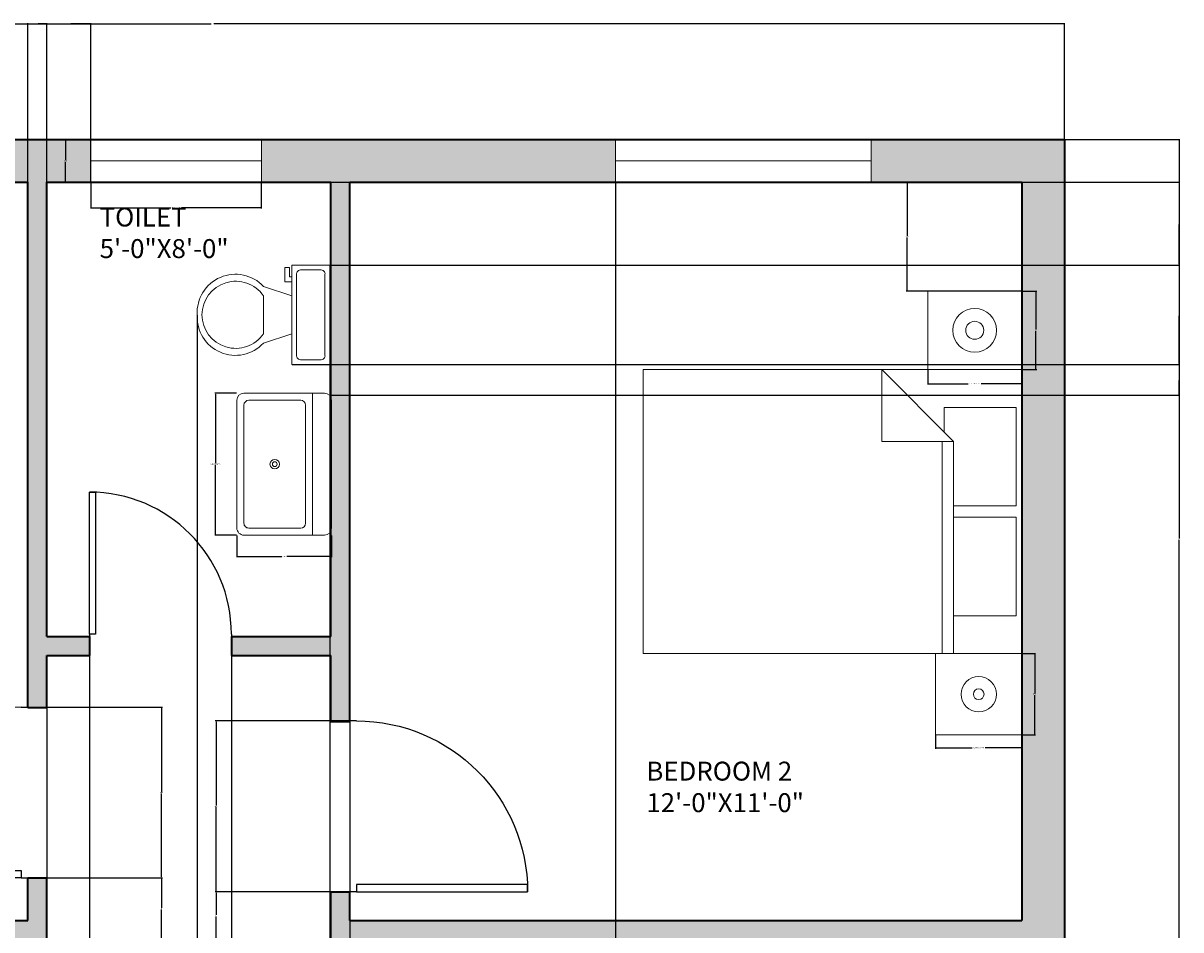
# Model space of a CAD drawing. Units: inches. Extents: x -29 to 443, y -589 to 39.
# Tile 5 of 5: x 139 to 384, y -153 to 39. Entities that reach past the tile are written whole.
import ezdxf

# ---------------------------------------------------------------- set-up
doc = ezdxf.new("R2010")
doc.units = ezdxf.units.IN
for name, color, linetype, lineweight in [('A-ANNO-DIMS', 2, 'Continuous', 18), ('A-AREA-IDEN', 7, 'Continuous', 18), ('A-DOOR', 3, 'Continuous', 25), ('A-FLOR-FIXT', 9, 'Continuous', 18), ('A-FURN', 9, 'Continuous', 18), ('A-GLAZ', 4, 'Continuous', 18), ('A-WALL', 7, 'Continuous', 35)]:
    doc.layers.add(name, color=color, linetype=linetype, lineweight=lineweight)
doc.layers.add('A-WALL-PATT', color=251, linetype='Continuous', lineweight=13, true_color=0x636466)
doc.styles.get("Standard").update_dxf_attribs({"font": 'arial.ttf'})
doc.dimstyles.get("Standard").update_dxf_attribs({"dimtxt": 0.18, "dimasz": 0.18, "dimexe": 0.18, "dimexo": 0.0625, "dimgap": 0.09, "dimtad": 0, "dimtih": 1, "dimtoh": 1, "dimdec": 4, "dimzin": 0, "dimdsep": 46, "dimtxsty": 'Standard', "dimcen": 0.09, "dimadec": 0, "dimazin": 0, "dimtfac": 1, "dimtdec": 4, "dimtofl": 0, "dimtmove": 0, "dimatfit": 3, "dimfxl": 1, "dimtolj": 1, "dimtzin": 0, "dimarcsym": 0})

# ---------------------------------------------------------------- blocks, each defined once
blk = doc.blocks.new('*U3')
for p, q in [((0, 0), (0, -6)), ((40, 0), (40, -6))]:
    blk.add_line(p, q)
blk.add_lwpolyline([(0, 0), (0, 40), (1.75, 40), (1.75, 0)], close=True)
blk.add_arc((0, 0), 40, 0, 90)
blk = doc.blocks.new('Sink-single - 30 in top')
blk.add_line((-15, -3.999996), (15, -3.999996))
for points in [[(-13.5, 0), (13.5, 0)], [(-15, -18.499996), (-15, -1.5)], [(15, -1.5), (15, -18.499996)], [(-13.5, -17.499996), (-13.5, -6.499996)], [(-12.5, -5.499996), (12.5, -5.499996)], [(13.5, -6.499996), (13.5, -17.499996)], [(12.5, -18.499996), (-12.5, -18.499996)], [(13.5, -19.999996), (-13.5, -19.999996)]]:
    blk.add_lwpolyline(points)
for radius in [1, 0.5]:
    blk.add_circle((0, -11.999996), radius)
for centre, radius, start, end in [((-13.5, -1.5), 1.5, 90, 180), ((13.5, -1.5), 1.5, 0, 90), ((-12.5, -6.499996), 1, 90, 180), ((12.5, -6.499996), 1, 0, 90), ((-13.5, -18.499996), 1.5, 180, 270), ((-12.5, -17.499996), 1, 180, 270), ((12.5, -17.499996), 1, 270, 0), ((13.5, -18.499996), 1.5, 270, 0)]:
    blk.add_arc(centre, radius, start, end)
blk = doc.blocks.new('Bed - Queen')
for p, q in [((0, -80.00003), (0, 0)), ((0, 0), (59.99999, 0)), ((59.99999, 0), (59.99999, -80.00003)), ((7.99999, -1.2), (28.79998, -1.2)), ((7.99999, -14.4), (7.99999, -1.2)), ((28.79998, -1.2), (28.79998, -14.4)), ((31.19999, -1.2), (51.99999, -1.2)), ((31.19999, -14.4), (31.19999, -1.2)), ((51.99999, -1.2), (51.99999, -16.4)), ((0, -14.4), (44.8, -14.4)), ((59.99999, -29.6), (44.8, -14.4)), ((44.8, -14.4), (44.8, -29.6)), ((44.8, -16.8), (0, -16.8)), ((51.99999, -16.4), (46.79936, -16.4)), ((44.8, -29.6), (59.99999, -29.6)), ((59.99999, -80.00003), (0, -80.00003))]:
    blk.add_line(p, q)
blk = doc.blocks.new('*U9')
for p, q in [((9.5, -6), (9.5, -2)), ((-10, -8.5), (-8, -8.5)), ((-10, -9.5), (-10, -8.5)), ((-7, -9.5), (-10, -9.5)), ((-8, -8.5), (-8, -8)), ((-7, -8), (-7, -9.5)), ((-4, -8), (-6, -14)), ((4, -8), (6, -14)), ((4, -14), (-4, -14))]:
    blk.add_line(p, q)
blk.add_lwpolyline([(10.5, -8), (10.5, 0), (-10.5, 0), (-10.5, -8)], close=True)
for points in [[(-9.5, -2), (-9.5, -6)], [(8.5, -1), (-8.5, -1)], [(-8.5, -7), (8.5, -7)]]:
    blk.add_lwpolyline(points)
for centre, radius, start, end in [((-8.625, -1.875), 0.8839, 81.8699, 188.1301), ((8.625, -1.875), 0.8839, 351.8699, 98.1301), ((-8.625, -6.125), 0.8839, 171.869898, 278.1301), ((8.625, -6.125), 0.8839, 261.8699, 8.1301), ((-0.4772, -19.9188), 8.0953, 133.01722, 273.38), ((0.0374, -19.8731), 7.127, 124.50543, 269.7), ((-0.0373, -19.8731), 7.127, 270.3, 55.4946), ((0.4773, -19.9188), 8.0953, 266.62, 46.9828)]:
    blk.add_arc(centre, radius, start, end)
blk = doc.blocks.new('WIN-54IN')
blk.add_line((54, 4.5), (0, 4.5))
blk.add_lwpolyline([(0, 9), (54, 9), (54, 0), (0, 0)], close=True)
blk = doc.blocks.new('WIN-36IN')
blk.add_line((4.5, 36), (4.5, 0))
blk.add_lwpolyline([(0, 0), (0, 36), (9, 36), (9, 0)], close=True)
blk = doc.blocks.new('NIGHTSTAND-LARGE')
blk.add_lwpolyline([(19.87, 0), (19.87, 16.61), (0, 16.61), (0, 0)], close=True)
for radius in [4.62, 1.9]:
    blk.add_circle((9.93, 8.31), radius)
blk = doc.blocks.new('NIGHTSTAND-SMALL')
blk.add_lwpolyline([(18.21, 17.2), (18.21, 0), (0, 0), (0, 17.2)], close=True)
for radius in [3.74, 1.13]:
    blk.add_circle((9.11, 8.6), radius)
blk = doc.blocks.new('*D22')
at = {"layer": 'A-ANNO-DIMS', "color": 0, "lineweight": -2, "transparency": 16777216}
for p, q in [((330.57, -34.29), (330.57, -37.39)), ((350.44, -34.29), (350.44, -37.39)), ((330.75, -37.21), (339.13, -37.21)), ((350.26, -37.21), (341.88, -37.21))]:
    blk.add_line(p, q, dxfattribs=at)
at = {"layer": 'A-ANNO-DIMS', "color": 0, "transparency": 16777216}
for points in [[(330.75, -37.18), (330.75, -37.24), (330.57, -37.21)], [(350.26, -37.18), (350.26, -37.24), (350.44, -37.21)]]:
    blk.add_solid(points, dxfattribs=at)
at = {"layer": 'Defpoints', "color": 0, "transparency": 16777216}
for p in [(330.57, -34.23), (350.44, -34.23), (350.44, -37.21)]:
    blk.add_point(p, dxfattribs=at)
at = {"layer": 'A-ANNO-DIMS', "color": 0, "transparency": 16777216, "insert": (340.5, -37.21), "char_height": 0.18, "attachment_point": 5}
blk.add_mtext('\\A1;NIGHTSTAND 20 TYP.', dxfattribs=at)
blk = doc.blocks.new('*D23')
at = {"layer": 'A-ANNO-DIMS', "color": 0, "lineweight": -2, "transparency": 16777216}
for p, q in [((350.5, -17.62), (353.6, -17.62)), ((353.42, -17.8), (353.42, -25.75)), ((353.42, -34.05), (353.42, -26.11)), ((350.5, -34.23), (353.6, -34.23))]:
    blk.add_line(p, q, dxfattribs=at)
at = {"layer": 'A-ANNO-DIMS', "color": 0, "transparency": 16777216}
for points in [[(353.39, -17.8), (353.45, -17.8), (353.42, -17.62)], [(353.39, -34.05), (353.45, -34.05), (353.42, -34.23)]]:
    blk.add_solid(points, dxfattribs=at)
at = {"layer": 'Defpoints', "color": 0, "transparency": 16777216}
for p in [(350.44, -17.62), (353.42, -17.62), (350.44, -34.23)]:
    blk.add_point(p, dxfattribs=at)
at = {"layer": 'A-ANNO-DIMS', "color": 0, "transparency": 16777216, "insert": (353.42, -25.93), "char_height": 0.18, "attachment_point": 5}
blk.add_mtext('\\A1;17 TYP.', dxfattribs=at)
blk = doc.blocks.new('*D24')
at = {"layer": 'A-ANNO-DIMS', "color": 0, "lineweight": -2, "transparency": 16777216}
for p, q in [((332.22, -111.49), (332.22, -114.34)), ((350.44, -111.49), (350.44, -114.34)), ((332.4, -114.16), (339.95, -114.16)), ((350.26, -114.16), (342.7, -114.16))]:
    blk.add_line(p, q, dxfattribs=at)
at = {"layer": 'A-ANNO-DIMS', "color": 0, "transparency": 16777216}
for points in [[(332.4, -114.13), (332.4, -114.19), (332.22, -114.16)], [(350.26, -114.13), (350.26, -114.19), (350.44, -114.16)]]:
    blk.add_solid(points, dxfattribs=at)
at = {"layer": 'Defpoints', "color": 0, "transparency": 16777216}
for p in [(332.22, -111.43), (350.44, -111.43), (350.44, -114.16)]:
    blk.add_point(p, dxfattribs=at)
at = {"layer": 'A-ANNO-DIMS', "color": 0, "transparency": 16777216, "insert": (341.33, -114.16), "char_height": 0.18, "attachment_point": 5}
blk.add_mtext('\\A1;NIGHTSTAND 18 TYP.', dxfattribs=at)
blk = doc.blocks.new('*D25')
at = {"layer": 'A-ANNO-DIMS', "color": 0, "lineweight": -2, "transparency": 16777216}
for p, q in [((350.5, -94.23), (353.35, -94.23)), ((353.17, -94.41), (353.17, -102.65)), ((353.17, -111.25), (353.17, -103.01)), ((350.5, -111.43), (353.35, -111.43))]:
    blk.add_line(p, q, dxfattribs=at)
at = {"layer": 'A-ANNO-DIMS', "color": 0, "transparency": 16777216}
for points in [[(353.14, -94.41), (353.2, -94.41), (353.17, -94.23)], [(353.14, -111.25), (353.2, -111.25), (353.17, -111.43)]]:
    blk.add_solid(points, dxfattribs=at)
at = {"layer": 'Defpoints', "color": 0, "transparency": 16777216}
for p in [(350.44, -94.23), (353.17, -94.23), (350.44, -111.43)]:
    blk.add_point(p, dxfattribs=at)
at = {"layer": 'A-ANNO-DIMS', "color": 0, "transparency": 16777216, "insert": (353.17, -102.83), "char_height": 0.18, "attachment_point": 5}
blk.add_mtext('\\A1;17 TYP.', dxfattribs=at)
blk = doc.blocks.new('*D26')
at = {"layer": 'A-ANNO-DIMS', "color": 0, "lineweight": -2, "transparency": 16777216}
for p, q in [((184.53, -39.21), (179.91, -39.21)), ((180.09, -39.39), (180.09, -54.03)), ((180.09, -69.03), (180.09, -54.39)), ((184.53, -69.21), (179.91, -69.21))]:
    blk.add_line(p, q, dxfattribs=at)
at = {"layer": 'A-ANNO-DIMS', "color": 0, "transparency": 16777216}
for points in [[(180.06, -39.39), (180.12, -39.39), (180.09, -39.21)], [(180.06, -69.03), (180.12, -69.03), (180.09, -69.21)]]:
    blk.add_solid(points, dxfattribs=at)
at = {"layer": 'Defpoints', "color": 0, "transparency": 16777216}
for p in [(184.59, -39.21), (180.09, -69.21), (184.59, -69.21)]:
    blk.add_point(p, dxfattribs=at)
at = {"layer": 'A-ANNO-DIMS', "color": 0, "transparency": 16777216, "insert": (180.09, -54.21), "char_height": 0.18, "attachment_point": 5}
blk.add_mtext('\\A1;BASIN TOP 30 TYP.', dxfattribs=at)
blk = doc.blocks.new('*D27')
at = {"layer": 'A-ANNO-DIMS', "color": 0, "lineweight": -2, "transparency": 16777216}
for p, q in [((184.59, -69.27), (184.59, -73.89)), ((204.59, -69.27), (204.59, -73.89)), ((184.77, -73.71), (194.06, -73.71)), ((204.41, -73.71), (195.12, -73.71))]:
    blk.add_line(p, q, dxfattribs=at)
at = {"layer": 'A-ANNO-DIMS', "color": 0, "transparency": 16777216}
for points in [[(184.77, -73.68), (184.77, -73.74), (184.59, -73.71)], [(204.41, -73.68), (204.41, -73.74), (204.59, -73.71)]]:
    blk.add_solid(points, dxfattribs=at)
at = {"layer": 'Defpoints', "color": 0, "transparency": 16777216}
for p in [(184.59, -69.21), (204.59, -69.21), (204.59, -73.71)]:
    blk.add_point(p, dxfattribs=at)
at = {"layer": 'A-ANNO-DIMS', "color": 0, "transparency": 16777216, "insert": (194.59, -73.71), "char_height": 0.18, "attachment_point": 5}
blk.add_mtext('\\A1;20 TYP.', dxfattribs=at)
blk = doc.blocks.new('*D28')
at = {"layer": 'A-ANNO-DIMS', "color": 0, "lineweight": -2, "transparency": 16777216}
for p, q in [((153.76, 5.32), (153.76, -0.19)), ((189.76, 5.32), (189.76, -0.19)), ((153.94, -0.01), (170.64, -0.01)), ((189.58, -0.01), (172.88, -0.01))]:
    blk.add_line(p, q, dxfattribs=at)
at = {"layer": 'A-ANNO-DIMS', "color": 0, "transparency": 16777216}
for points in [[(153.94, 0.02), (153.94, -0.04), (153.76, -0.01)], [(189.58, 0.02), (189.58, -0.04), (189.76, -0.01)]]:
    blk.add_solid(points, dxfattribs=at)
at = {"layer": 'Defpoints', "color": 0, "transparency": 16777216}
for p in [(153.76, 5.39), (189.76, 5.39), (189.76, -0.01)]:
    blk.add_point(p, dxfattribs=at)
at = {"layer": 'A-ANNO-DIMS', "color": 0, "transparency": 16777216, "insert": (171.76, -0.01), "char_height": 0.18, "attachment_point": 5}
blk.add_mtext('\\A1;WINDOW 36 TYP.', dxfattribs=at)
blk = doc.blocks.new('*D29')
at = {"layer": 'A-ANNO-DIMS', "color": 0, "lineweight": -2, "transparency": 16777216}
for p, q in [((153.7, 14.39), (148.18, 14.39)), ((148.36, 14.21), (148.36, 10.07)), ((148.36, 5.57), (148.36, 9.7)), ((153.7, 5.39), (148.18, 5.39))]:
    blk.add_line(p, q, dxfattribs=at)
at = {"layer": 'A-ANNO-DIMS', "color": 0, "transparency": 16777216}
for points in [[(148.33, 14.21), (148.39, 14.21), (148.36, 14.39)], [(148.33, 5.57), (148.39, 5.57), (148.36, 5.39)]]:
    blk.add_solid(points, dxfattribs=at)
at = {"layer": 'Defpoints', "color": 0, "transparency": 16777216}
for p in [(153.76, 14.39), (148.36, 5.39), (153.76, 5.39)]:
    blk.add_point(p, dxfattribs=at)
at = {"layer": 'A-ANNO-DIMS', "color": 0, "transparency": 16777216, "insert": (148.36, 9.89), "char_height": 0.18, "attachment_point": 5}
blk.add_mtext('\\A1;9 TYP.', dxfattribs=at)
blk = doc.blocks.new('*D36')
at = {"layer": 'A-ANNO-DIMS', "color": 0, "lineweight": -2, "transparency": 16777216}
for p, q in [((-0.56, 14.45), (-0.56, 38.99)), ((-0.38, 38.81), (179.15, 38.81)), ((359.26, 38.81), (179.72, 38.81)), ((359.44, 14.45), (359.44, 38.99))]:
    blk.add_line(p, q, dxfattribs=at)
at = {"layer": 'A-ANNO-DIMS', "color": 0, "transparency": 16777216}
for points in [[(-0.38, 38.84), (-0.38, 38.78), (-0.56, 38.81)], [(359.26, 38.84), (359.26, 38.78), (359.44, 38.81)]]:
    blk.add_solid(points, dxfattribs=at)
at = {"layer": 'Defpoints', "color": 0, "transparency": 16777216}
for p in [(359.44, 38.81), (-0.56, 14.39), (359.44, 14.39)]:
    blk.add_point(p, dxfattribs=at)
at = {"layer": 'A-ANNO-DIMS', "color": 0, "transparency": 16777216, "insert": (179.44, 38.81), "char_height": 0.18, "attachment_point": 5}
blk.add_mtext('\\A1;360', dxfattribs=at)
blk = doc.blocks.new('*D39')
at = {"layer": 'A-ANNO-DIMS', "color": 0, "lineweight": -2, "transparency": 16777216}
for p, q in [((144.44, 5.45), (144.44, 38.99)), ((144.62, 38.81), (148.71, 38.81)), ((153.58, 38.81), (149.49, 38.81)), ((153.76, 5.45), (153.76, 38.99))]:
    blk.add_line(p, q, dxfattribs=at)
at = {"layer": 'A-ANNO-DIMS', "color": 0, "transparency": 16777216}
for points in [[(144.62, 38.84), (144.62, 38.78), (144.44, 38.81)], [(153.58, 38.84), (153.58, 38.78), (153.76, 38.81)]]:
    blk.add_solid(points, dxfattribs=at)
at = {"layer": 'Defpoints', "color": 0, "transparency": 16777216}
for p in [(144.44, 38.81), (144.44, 5.39), (153.76, 5.39)]:
    blk.add_point(p, dxfattribs=at)
at = {"layer": 'A-ANNO-DIMS', "color": 0, "transparency": 16777216, "insert": (149.1, 38.81), "char_height": 0.18, "attachment_point": 5}
blk.add_mtext('\\A1;9.326', dxfattribs=at)
blk = doc.blocks.new('*D40')
at = {"layer": 'A-ANNO-DIMS', "color": 0, "lineweight": -2, "transparency": 16777216}
for p, q in [((208.44, 5.32), (208.44, -492.89)), ((264.58, 5.32), (264.58, -492.89)), ((208.62, -492.71), (236.11, -492.71)), ((264.4, -492.71), (236.9, -492.71))]:
    blk.add_line(p, q, dxfattribs=at)
at = {"layer": 'A-ANNO-DIMS', "color": 0, "transparency": 16777216}
for points in [[(208.62, -492.68), (208.62, -492.74), (208.44, -492.71)], [(264.4, -492.68), (264.4, -492.74), (264.58, -492.71)]]:
    blk.add_solid(points, dxfattribs=at)
at = {"layer": 'Defpoints', "color": 0, "transparency": 16777216}
for p in [(208.44, 5.39), (264.58, 5.39), (208.44, -492.71)]:
    blk.add_point(p, dxfattribs=at)
at = {"layer": 'A-ANNO-DIMS', "color": 0, "transparency": 16777216, "insert": (236.51, -492.71), "char_height": 0.18, "attachment_point": 5}
blk.add_mtext('\\A1;56.14', dxfattribs=at)
blk = doc.blocks.new('*D44')
at = {"layer": 'A-ANNO-DIMS', "color": 0, "lineweight": -2, "transparency": 16777216}
for p, q in [((359.5, 14.39), (383.85, 14.39)), ((383.67, 14.21), (383.67, -69.93)), ((383.67, -154.43), (383.67, -70.3)), ((359.5, -154.61), (383.85, -154.61))]:
    blk.add_line(p, q, dxfattribs=at)
at = {"layer": 'A-ANNO-DIMS', "color": 0, "transparency": 16777216}
for points in [[(383.64, 14.21), (383.7, 14.21), (383.67, 14.39)], [(383.64, -154.43), (383.7, -154.43), (383.67, -154.61)]]:
    blk.add_solid(points, dxfattribs=at)
at = {"layer": 'Defpoints', "color": 0, "transparency": 16777216}
for p in [(359.44, 14.39), (359.44, -154.61), (383.67, -154.61)]:
    blk.add_point(p, dxfattribs=at)
at = {"layer": 'A-ANNO-DIMS', "color": 0, "transparency": 16777216, "insert": (383.67, -70.11), "char_height": 0.18, "attachment_point": 5}
blk.add_mtext('\\A1;169', dxfattribs=at)
blk = doc.blocks.new('*D50')
at = {"layer": 'A-ANNO-DIMS', "color": 0, "lineweight": -2, "transparency": 16777216}
for p, q in [((144.5, -105.59), (168.85, -105.59)), ((168.67, -105.77), (168.67, -123.42)), ((168.67, -141.43), (168.67, -123.78)), ((144.5, -141.61), (168.85, -141.61))]:
    blk.add_line(p, q, dxfattribs=at)
at = {"layer": 'A-ANNO-DIMS', "color": 0, "transparency": 16777216}
for points in [[(168.64, -105.77), (168.7, -105.77), (168.67, -105.59)], [(168.64, -141.43), (168.7, -141.43), (168.67, -141.61)]]:
    blk.add_solid(points, dxfattribs=at)
at = {"layer": 'Defpoints', "color": 0, "transparency": 16777216}
for p in [(144.44, -105.59), (144.44, -141.61), (168.67, -141.61)]:
    blk.add_point(p, dxfattribs=at)
at = {"layer": 'A-ANNO-DIMS', "color": 0, "transparency": 16777216, "insert": (168.67, -123.6), "char_height": 0.18, "attachment_point": 5}
blk.add_mtext('\\A1;36.03', dxfattribs=at)
blk = doc.blocks.new('*D51')
at = {"layer": 'A-ANNO-DIMS', "color": 0, "lineweight": -2, "transparency": 16777216}
for p, q in [((144.5, -141.61), (168.85, -141.61)), ((168.67, -141.79), (168.67, -147.93)), ((168.67, -154.43), (168.67, -148.3)), ((144.5, -154.61), (168.85, -154.61))]:
    blk.add_line(p, q, dxfattribs=at)
at = {"layer": 'A-ANNO-DIMS', "color": 0, "transparency": 16777216}
for points in [[(168.64, -141.79), (168.7, -141.79), (168.67, -141.61)], [(168.64, -154.43), (168.7, -154.43), (168.67, -154.61)]]:
    blk.add_solid(points, dxfattribs=at)
at = {"layer": 'Defpoints', "color": 0, "transparency": 16777216}
for p in [(144.44, -141.61), (144.44, -154.61), (168.67, -154.61)]:
    blk.add_point(p, dxfattribs=at)
at = {"layer": 'A-ANNO-DIMS', "color": 0, "transparency": 16777216, "insert": (168.67, -148.11), "char_height": 0.18, "attachment_point": 5}
blk.add_mtext('\\A1;13', dxfattribs=at)
blk = doc.blocks.new('*D52')
at = {"layer": 'A-ANNO-DIMS', "color": 0, "lineweight": -2, "transparency": 16777216}
for p, q in [((153.44, -94.68), (153.44, -492.89)), ((183.44, -94.68), (183.44, -492.89)), ((153.62, -492.71), (168.22, -492.71)), ((183.26, -492.71), (168.65, -492.71))]:
    blk.add_line(p, q, dxfattribs=at)
at = {"layer": 'A-ANNO-DIMS', "color": 0, "transparency": 16777216}
for points in [[(153.62, -492.68), (153.62, -492.74), (153.44, -492.71)], [(183.26, -492.68), (183.26, -492.74), (183.44, -492.71)]]:
    blk.add_solid(points, dxfattribs=at)
at = {"layer": 'Defpoints', "color": 0, "transparency": 16777216}
for p in [(153.44, -94.61), (183.44, -94.61), (183.44, -492.71)]:
    blk.add_point(p, dxfattribs=at)
at = {"layer": 'A-ANNO-DIMS', "color": 0, "transparency": 16777216, "insert": (168.44, -492.71), "char_height": 0.18, "attachment_point": 5}
blk.add_mtext('\\A1;30', dxfattribs=at)
blk = doc.blocks.new('*D62')
at = {"layer": 'A-ANNO-DIMS', "color": 0, "lineweight": -2, "transparency": 16777216}
for p, q in [((204.37, -108.46), (180.03, -108.46)), ((180.21, -108.64), (180.21, -126.36)), ((180.21, -144.43), (180.21, -126.72)), ((204.37, -144.61), (180.03, -144.61))]:
    blk.add_line(p, q, dxfattribs=at)
at = {"layer": 'A-ANNO-DIMS', "color": 0, "transparency": 16777216}
for points in [[(180.18, -108.64), (180.24, -108.64), (180.21, -108.46)], [(180.18, -144.43), (180.24, -144.43), (180.21, -144.61)]]:
    blk.add_solid(points, dxfattribs=at)
at = {"layer": 'Defpoints', "color": 0, "transparency": 16777216}
for p in [(180.21, -108.46), (204.44, -108.46), (204.44, -144.61)]:
    blk.add_point(p, dxfattribs=at)
at = {"layer": 'A-ANNO-DIMS', "color": 0, "transparency": 16777216, "insert": (180.21, -126.54), "char_height": 0.18, "attachment_point": 5}
blk.add_mtext('\\A1;36.15', dxfattribs=at)
blk = doc.blocks.new('*D63')
at = {"layer": 'A-ANNO-DIMS', "color": 0, "lineweight": -2, "transparency": 16777216}
for p, q in [((204.37, -144.61), (180.03, -144.61)), ((180.21, -144.79), (180.21, -149.43)), ((180.21, -154.43), (180.21, -149.8)), ((204.37, -154.61), (180.03, -154.61))]:
    blk.add_line(p, q, dxfattribs=at)
at = {"layer": 'A-ANNO-DIMS', "color": 0, "transparency": 16777216}
for points in [[(180.18, -144.79), (180.24, -144.79), (180.21, -144.61)], [(180.18, -154.43), (180.24, -154.43), (180.21, -154.61)]]:
    blk.add_solid(points, dxfattribs=at)
at = {"layer": 'Defpoints', "color": 0, "transparency": 16777216}
for p in [(180.21, -144.61), (204.44, -144.61), (204.44, -154.61)]:
    blk.add_point(p, dxfattribs=at)
at = {"layer": 'A-ANNO-DIMS', "color": 0, "transparency": 16777216, "insert": (180.21, -149.61), "char_height": 0.18, "attachment_point": 5}
blk.add_mtext('\\A1;10', dxfattribs=at)
blk = doc.blocks.new('*D67')
at = {"layer": 'A-ANNO-DIMS', "color": 0, "lineweight": -2, "transparency": 16777216}
for p, q in [((204.5, 5.39), (383.85, 5.39)), ((383.67, 5.21), (383.67, -3.2)), ((383.67, -11.97), (383.67, -3.56)), ((204.27, -12.15), (383.85, -12.15))]:
    blk.add_line(p, q, dxfattribs=at)
at = {"layer": 'A-ANNO-DIMS', "color": 0, "transparency": 16777216}
for points in [[(383.64, 5.21), (383.7, 5.21), (383.67, 5.39)], [(383.64, -11.97), (383.7, -11.97), (383.67, -12.15)]]:
    blk.add_solid(points, dxfattribs=at)
at = {"layer": 'Defpoints', "color": 0, "transparency": 16777216}
for p in [(204.44, 5.39), (204.21, -12.15), (383.67, -12.15)]:
    blk.add_point(p, dxfattribs=at)
at = {"layer": 'A-ANNO-DIMS', "color": 0, "transparency": 16777216, "insert": (383.67, -3.38), "char_height": 0.18, "attachment_point": 5}
blk.add_mtext('\\A1;17.533', dxfattribs=at)
blk = doc.blocks.new('*D68')
at = {"layer": 'A-ANNO-DIMS', "color": 0, "lineweight": -2, "transparency": 16777216}
for p, q in [((176.21, -22.71), (176.21, -492.89)), ((204.21, -33.21), (204.21, -492.89)), ((176.39, -492.71), (189.99, -492.71)), ((204.03, -492.71), (190.43, -492.71))]:
    blk.add_line(p, q, dxfattribs=at)
at = {"layer": 'A-ANNO-DIMS', "color": 0, "transparency": 16777216}
for points in [[(176.39, -492.68), (176.39, -492.74), (176.21, -492.71)], [(204.03, -492.68), (204.03, -492.74), (204.21, -492.71)]]:
    blk.add_solid(points, dxfattribs=at)
at = {"layer": 'Defpoints', "color": 0, "transparency": 16777216}
for p in [(176.21, -22.65), (204.21, -33.15), (204.21, -492.71)]:
    blk.add_point(p, dxfattribs=at)
at = {"layer": 'A-ANNO-DIMS', "color": 0, "transparency": 16777216, "insert": (190.21, -492.71), "char_height": 0.18, "attachment_point": 5}
blk.add_mtext('\\A1;28', dxfattribs=at)
blk = doc.blocks.new('*D69')
at = {"layer": 'A-ANNO-DIMS', "color": 0, "lineweight": -2, "transparency": 16777216}
for p, q in [((204.27, -12.15), (383.85, -12.15)), ((383.67, -12.33), (383.67, -22.47)), ((383.67, -32.97), (383.67, -22.83)), ((204.27, -33.15), (383.85, -33.15))]:
    blk.add_line(p, q, dxfattribs=at)
at = {"layer": 'A-ANNO-DIMS', "color": 0, "transparency": 16777216}
for points in [[(383.64, -12.33), (383.7, -12.33), (383.67, -12.15)], [(383.64, -32.97), (383.7, -32.97), (383.67, -33.15)]]:
    blk.add_solid(points, dxfattribs=at)
at = {"layer": 'Defpoints', "color": 0, "transparency": 16777216}
for p in [(204.21, -12.15), (383.67, -12.15), (204.21, -33.15)]:
    blk.add_point(p, dxfattribs=at)
at = {"layer": 'A-ANNO-DIMS', "color": 0, "transparency": 16777216, "insert": (383.67, -22.65), "char_height": 0.18, "attachment_point": 5}
blk.add_mtext('\\A1;21', dxfattribs=at)
blk = doc.blocks.new('*D70')
at = {"layer": 'A-ANNO-DIMS', "color": 0, "lineweight": -2, "transparency": 16777216}
for p, q in [((196.27, -33.15), (383.85, -33.15)), ((383.67, -33.33), (383.67, -36.22)), ((383.67, -39.47), (383.67, -36.58)), ((204.21, -39.65), (383.85, -39.65))]:
    blk.add_line(p, q, dxfattribs=at)
at = {"layer": 'A-ANNO-DIMS', "color": 0, "transparency": 16777216}
for points in [[(383.64, -33.33), (383.7, -33.33), (383.67, -33.15)], [(383.64, -39.47), (383.7, -39.47), (383.67, -39.65)]]:
    blk.add_solid(points, dxfattribs=at)
at = {"layer": 'Defpoints', "color": 0, "transparency": 16777216}
for p in [(196.21, -33.15), (204.15, -39.65), (383.67, -39.65)]:
    blk.add_point(p, dxfattribs=at)
at = {"layer": 'A-ANNO-DIMS', "color": 0, "transparency": 16777216, "insert": (383.67, -36.4), "char_height": 0.18, "attachment_point": 5}
blk.add_mtext('\\A1;6.5', dxfattribs=at)
blk = doc.blocks.new('*D71')
at = {"layer": 'A-ANNO-DIMS', "color": 0, "lineweight": -2, "transparency": 16777216}
for p, q in [((144.44, -94.68), (144.44, -492.89)), ((153.44, -94.68), (153.44, -492.89)), ((144.62, -492.71), (148.79, -492.71)), ((153.26, -492.71), (149.09, -492.71))]:
    blk.add_line(p, q, dxfattribs=at)
at = {"layer": 'A-ANNO-DIMS', "color": 0, "transparency": 16777216}
for points in [[(144.62, -492.68), (144.62, -492.74), (144.44, -492.71)], [(153.26, -492.68), (153.26, -492.74), (153.44, -492.71)]]:
    blk.add_solid(points, dxfattribs=at)
at = {"layer": 'Defpoints', "color": 0, "transparency": 16777216}
for p in [(144.44, -94.61), (153.44, -94.61), (153.44, -492.71)]:
    blk.add_point(p, dxfattribs=at)
at = {"layer": 'A-ANNO-DIMS', "color": 0, "transparency": 16777216, "insert": (148.94, -492.71), "char_height": 0.18, "attachment_point": 5}
blk.add_mtext('\\A1;9', dxfattribs=at)
blk = doc.blocks.new('*D72')
at = {"layer": 'A-ANNO-DIMS', "color": 0, "lineweight": -2, "transparency": 16777216}
for p, q in [((140.44, 5.45), (140.44, 38.99)), ((140.62, 38.81), (142.28, 38.81)), ((144.26, 38.81), (142.59, 38.81)), ((144.44, 5.45), (144.44, 38.99))]:
    blk.add_line(p, q, dxfattribs=at)
at = {"layer": 'A-ANNO-DIMS', "color": 0, "transparency": 16777216}
for points in [[(140.62, 38.84), (140.62, 38.78), (140.44, 38.81)], [(144.26, 38.84), (144.26, 38.78), (144.44, 38.81)]]:
    blk.add_solid(points, dxfattribs=at)
at = {"layer": 'Defpoints', "color": 0, "transparency": 16777216}
for p in [(144.44, 38.81), (140.44, 5.39), (144.44, 5.39)]:
    blk.add_point(p, dxfattribs=at)
at = {"layer": 'A-ANNO-DIMS', "color": 0, "transparency": 16777216, "insert": (142.44, 38.81), "char_height": 0.18, "attachment_point": 5}
blk.add_mtext('\\A1;4', dxfattribs=at)
blk = doc.blocks.new('*D80')
at = {"layer": 'A-ANNO-DIMS', "color": 0, "lineweight": -2, "transparency": 16777216}
for p, q in [((350.37, 5.39), (326.03, 5.39)), ((326.21, 5.21), (326.21, -5.94)), ((326.21, -17.44), (326.21, -6.3)), ((350.37, -17.62), (326.03, -17.62))]:
    blk.add_line(p, q, dxfattribs=at)
at = {"layer": 'A-ANNO-DIMS', "color": 0, "transparency": 16777216}
for points in [[(326.18, 5.21), (326.24, 5.21), (326.21, 5.39)], [(326.18, -17.44), (326.24, -17.44), (326.21, -17.62)]]:
    blk.add_solid(points, dxfattribs=at)
at = {"layer": 'Defpoints', "color": 0, "transparency": 16777216}
for p in [(326.21, 5.39), (350.44, 5.39), (350.44, -17.62)]:
    blk.add_point(p, dxfattribs=at)
at = {"layer": 'A-ANNO-DIMS', "color": 0, "transparency": 16777216, "insert": (326.21, -6.12), "char_height": 0.18, "attachment_point": 5}
blk.add_mtext('\\A1;23.006', dxfattribs=at)

msp = doc.modelspace()

# ---------------------------------------------------------------- hatches: boundary and pattern name
at = {"layer": 'A-WALL-PATT'}
h = msp.add_hatch(color=256, dxfattribs=at)
h.dxf.hatch_style = 1
h.paths.add_polyline_path([(8.4359, 5.3851), (38.6638, 5.3851), (38.6638, 14.3851), (-0.5641, 14.3851), (-0.5641, -161.7206), (8.4359, -161.7206), (8.4359, -154.6149), (98.4359, -154.6149), (98.4359, -169.6149), (102.4359, -169.6149), (102.4359, -154.6149), (144.4359, -154.6149), (144.4359, -141.6149), (140.4359, -141.6149), (140.4359, -150.6149), (8.4359, -150.6149)])
h.paths.add_polyline_path([(153.762, 14.3851), (92.6638, 14.3851), (92.6638, 5.3851), (140.4359, 5.3851), (140.4359, -105.5868), (144.4359, -105.5868), (144.4359, -94.6149), (153.4359, -94.6149), (153.4359, -90.6149), (144.4359, -90.6149), (144.4359, 5.3851), (153.762, 5.3851)])
h.paths.add_polyline_path([(264.576, 14.3851), (189.762, 14.3851), (189.762, 5.3851), (204.4359, 5.3851), (204.4359, -40.0486, -0.11439146), (204.5889, -40.7086), (204.5889, -67.7086, -0.11439146), (204.4359, -68.3685), (204.4359, -90.6149), (183.4359, -90.6149), (183.4359, -94.6149), (204.4359, -94.6149), (204.4359, -108.4622), (208.4359, -108.4622), (208.4359, 5.3851), (264.576, 5.3851)])
h.paths.add_polyline_path([(359.4359, 14.3851), (318.576, 14.3851), (318.576, 5.3851), (350.4359, 5.3851), (350.4359, -150.6149), (208.4359, -150.6149), (208.4359, -144.6149), (204.4359, -144.6149), (204.4359, -154.6149), (286.4359, -154.6149), (286.4359, -169.4775), (290.4359, -169.4775), (290.4359, -154.6149), (359.4359, -154.6149)])
h.paths.add_polyline_path([(8.4359, -212.6149), (98.4359, -212.6149), (102.4359, -212.6149), (102.4359, -199.6149), (98.4359, -199.6149), (98.4359, -208.6149), (8.4359, -208.6149), (8.4359, -197.7206), (-0.5641, -197.7206), (-0.5641, -417.6149), (114.4359, -417.6149), (114.4359, -354.6149), (134.4359, -354.6149), (134.4359, -453.6149), (147.4359, -453.6149), (147.4359, -444.6149), (138.4359, -444.6149), (138.4359, -212.6149), (129.4359, -212.6149), (129.4359, -216.6149), (134.4359, -216.6149), (134.4359, -350.6149), (110.4359, -350.6149), (110.4359, -377.2063, -0.30395766), (111.1497, -378.2719, -0.30395766), (110.4359, -379.3376), (110.4359, -408.6149), (8.4359, -408.6149)])
h.paths.add_polyline_path([(265.0252, -444.6149), (230.4359, -444.6149), (230.4359, -396.6149), (246.223, -396.6149), (246.223, -392.6149), (230.4359, -392.6149), (230.4359, -302.6149), (245.4886, -302.6149), (245.4886, -298.6149), (226.4359, -298.6149), (226.4359, -444.6149), (189.4359, -444.6149), (189.4359, -453.6149), (226.4359, -453.6149), (265.0252, -453.6149)])
h.paths.add_polyline_path([(359.4359, -417.6149), (359.4359, -377.3771), (350.4359, -377.3771), (350.4359, -392.6149), (276.3235, -392.6149), (276.3235, -396.6149), (350.4359, -396.6149), (350.4359, -408.6149), (350.4359, -444.6149), (319.0252, -444.6149), (319.0252, -453.6149), (359.4359, -453.6149)])
h.paths.add_polyline_path([(359.4359, -298.6149), (290.4359, -298.6149), (290.4359, -289.6207), (286.4359, -289.6207), (286.4359, -298.6149), (277.8355, -298.6149), (277.8355, -302.6149), (350.4359, -302.6149), (350.4359, -323.3771), (359.4359, -323.3771)])
h.paths.add_polyline_path([(290.4359, -226.7916), (286.4359, -226.7916), (286.4359, -253.468), (290.4359, -253.468)])

# ---------------------------------------------------------------- linework, layer by layer
at = {"layer": 'A-WALL'}
for p, q in [((-0.5641, 14.3851), (359.4359, 14.3851)), ((359.4359, 14.3851), (359.4359, -154.6149)), ((8.4359, 5.3851), (140.4359, 5.3851)), ((140.4359, -105.6149), (140.4359, 5.3851)), ((144.4359, 5.3851), (204.4359, 5.3851)), ((144.4359, -90.6149), (144.4359, 5.3851)), ((204.4359, -90.6149), (204.4359, 5.3851)), ((208.4359, 5.3851), (350.4359, 5.3851)), ((208.4359, -108.6149), (208.4359, 5.3851)), ((350.4359, 5.3851), (350.4359, -150.6149)), ((144.4359, -90.6149), (153.4359, -90.6149)), ((153.4359, -90.6149), (153.4359, -94.6149)), ((183.4327, -90.6149), (204.4359, -90.6149)), ((183.4359, -90.6149), (183.4359, -94.6149)), ((144.4359, -94.6149), (153.4359, -94.6149)), ((144.4359, -105.6149), (144.4359, -94.6149)), ((183.4327, -94.6149), (204.4359, -94.6149)), ((204.4359, -108.6149), (204.4359, -94.6149)), ((140.4359, -105.6149), (144.4359, -105.6149)), ((204.4359, -108.6149), (208.4359, -108.6149)), ((140.4359, -150.6149), (140.4359, -141.6149)), ((140.4359, -141.6149), (144.4359, -141.6149)), ((144.4359, -154.6149), (144.4359, -141.6149)), ((204.4359, -154.6149), (204.4359, -144.6149)), ((204.4359, -144.6149), (208.4359, -144.6149)), ((208.4359, -150.6149), (208.4359, -144.6149)), ((8.4359, -150.6149), (140.4359, -150.6149)), ((208.4359, -150.6149), (350.4359, -150.6149))]:
    msp.add_line(p, q, dxfattribs=at)

# ---------------------------------------------------------------- block references
at = {"layer": 'A-DOOR', "xscale": 0.7499177992314163, "yscale": 0.7499177992314163, "zscale": 0.7499177992314163}
msp.add_blockref('*U3', (153.4359, -90.1154), dxfattribs=at)
at = {"layer": 'A-DOOR'}
for p, xscale, yscale, zscale, rotation in [((139.0317, -141.6149), 0.9007031816265564, 0.9007031816265564, 0.9007031816265564, 90), ((209.8589, -144.6149), -0.9038178546105021, 0.9038178546105021, 0.9038178546105021, 270)]:
    msp.add_blockref('*U3', p, dxfattribs=dict(at, xscale=xscale, yscale=yscale, zscale=zscale, rotation=rotation))
at = {"layer": 'A-FLOR-FIXT', "rotation": 270}
for name, p in [('*U9', (204.211, -22.6482)), ('Sink-single - 30 in top', (204.5889, -54.2086))]:
    msp.add_blockref(name, p, dxfattribs=at)
at = {"layer": 'A-FURN'}
for name, p in [('NIGHTSTAND-LARGE', (330.566, -34.232)), ('NIGHTSTAND-SMALL', (332.222, -111.428))]:
    msp.add_blockref(name, p, dxfattribs=at)
at = {"layer": 'A-FURN', "xscale": -1, "rotation": 270}
msp.add_blockref('Bed - Queen', (350.4359, -94.2324), dxfattribs=at)
at = {"layer": 'A-GLAZ', "rotation": 269.9999999999999}
msp.add_blockref('WIN-36IN', (153.7616, 14.3852), dxfattribs=at)
at = {"layer": 'A-GLAZ'}
msp.add_blockref('WIN-54IN', (264.5762, 5.3847), dxfattribs=at)

# ---------------------------------------------------------------- texts
at = {"layer": 'A-AREA-IDEN', "char_height": 4, "attachment_point": 1}
for s, width, insert in [('TOILET\\P5\'-0"X8\'-0"', 37.181232, (155.6029, 0.0141)), ('BEDROOM 2\\P12\'-0"X11\'-0"', 58.091895, (271.1183, -117.075))]:
    msp.add_mtext_dynamic_manual_height_columns(s, width=width, gutter_width=12.5, heights=[0], dxfattribs=dict(at, insert=insert))

# ---------------------------------------------------------------- dimensions: what is measured, and where the dimension line sits
at = {"layer": 'A-ANNO-DIMS'}
for base, p1, p2, override, picture, middle in [((359.4359, 38.8064), (-0.5641, 14.3851), (359.4359, 14.3851), {"dimdec": 0, "dimlfac": 1, "dimrnd": 0, "dimzin": 0, "dimdsep": 46, "dimlunit": 2}, '*D36', (179.4359, 38.8064)), ((144.4359, 38.8064), (140.4359, 5.3851), (144.4359, 5.3851), {"dimdec": 0, "dimlfac": 1, "dimrnd": 0, "dimzin": 0, "dimdsep": 46, "dimlunit": 2}, '*D72', (142.4359, 38.8064)), ((144.4359, 38.8064), (153.762, 5.3851), (144.4359, 5.3851), {"dimdec": 3, "dimlfac": 1, "dimrnd": 0, "dimzin": 0, "dimdsep": 46, "dimlunit": 2}, '*D39', (149.099, 38.8064)), ((208.4359, -492.7145), (264.576, 5.3851), (208.4359, 5.3851), {"dimdec": 2, "dimlfac": 1, "dimrnd": 0, "dimzin": 0, "dimdsep": 46, "dimlunit": 2}, '*D40', (236.506, -492.7145)), ((204.211, -492.7145), (176.211, -22.6482), (204.211, -33.1482), {"dimdec": 0, "dimlfac": 1, "dimrnd": 0, "dimzin": 0, "dimdsep": 46, "dimlunit": 2}, '*D68', (190.211, -492.7145)), ((153.4359, -492.7145), (144.4359, -94.6149), (153.4359, -94.6149), {"dimdec": 0, "dimlfac": 1, "dimrnd": 0, "dimzin": 0, "dimdsep": 46, "dimlunit": 2}, '*D71', (148.9359, -492.7145)), ((183.4359, -492.7145), (153.4359, -94.6149), (183.4359, -94.6149), {"dimdec": 0, "dimlfac": 1, "dimrnd": 0, "dimzin": 0, "dimdsep": 46, "dimlunit": 2}, '*D52', (168.4359, -492.7145))]:
    dim = msp.add_linear_dim(base=base, p1=p1, p2=p2, dimstyle='Standard', override=override, dxfattribs=at)
    dim.commit()
    dim.dimension.update_dxf_attribs({"geometry": picture, "text_midpoint": middle})
for base, p1, p2, angle, text, picture, middle in [((148.362, 5.3851), (153.762, 14.3851), (153.762, 5.3851), 270, '<> TYP.', '*D29', (148.362, 9.8851)), ((353.4164, -17.6208), (350.4359, -34.2324), (350.4359, -17.6208), 90, '<> TYP.', '*D23', (353.4164, -25.9266)), ((180.0889, -69.2086), (184.5889, -39.2086), (184.5889, -69.2086), 270, 'BASIN TOP <> TYP.', '*D26', (180.0889, -54.2086)), ((353.168, -94.2324), (350.4359, -111.4283), (350.4359, -94.2324), 90, '<> TYP.', '*D25', (353.168, -102.8304))]:
    dim = msp.add_linear_dim(base=base, p1=p1, p2=p2, angle=angle, text=text, dimstyle='Standard', override={"dimdec": 0, "dimlfac": 1, "dimrnd": 0, "dimzin": 0, "dimdsep": 46, "dimlunit": 2}, dxfattribs=at)
    dim.commit()
    dim.dimension.update_dxf_attribs({"geometry": picture, "text_midpoint": middle})
for base, p1, p2, angle, override, picture, middle in [((383.6659, -154.6149), (359.4359, 14.3851), (359.4359, -154.6149), 90, {"dimdec": 0, "dimlfac": 1, "dimrnd": 0, "dimzin": 0, "dimdsep": 46, "dimlunit": 2}, '*D44', (383.6659, -70.1149)), ((383.6659, -12.1482), (204.4359, 5.3851), (204.211, -12.1482), 90, {"dimdec": 3, "dimlfac": 1, "dimrnd": 0, "dimzin": 0, "dimdsep": 46, "dimlunit": 2}, '*D67', (383.6659, -3.3816)), ((326.2059, 5.3851), (350.4359, -17.6208), (350.4359, 5.3851), 90, {"dimdec": 3, "dimlfac": 1, "dimrnd": 0, "dimzin": 0, "dimdsep": 46, "dimlunit": 2}, '*D80', (326.2059, -6.1179)), ((383.6659, -12.1482), (204.211, -33.1482), (204.211, -12.1482), 90, {"dimdec": 0, "dimlfac": 1, "dimrnd": 0, "dimzin": 0, "dimdsep": 46, "dimlunit": 2}, '*D69', (383.6659, -22.6482)), ((383.6659, -39.6479), (196.211, -33.1482), (204.1496, -39.6479), 90, {"dimdec": 1, "dimlfac": 1, "dimrnd": 0, "dimzin": 0, "dimdsep": 46, "dimlunit": 2}, '*D70', (383.6659, -36.398)), ((168.6659, -141.6149), (144.4359, -105.5868), (144.4359, -141.6149), 270, {"dimdec": 2, "dimlfac": 1, "dimrnd": 0, "dimzin": 0, "dimdsep": 46, "dimlunit": 2}, '*D50', (168.6659, -123.6009)), ((180.2059, -108.4622), (204.4359, -144.6149), (204.4359, -108.4622), 90, {"dimdec": 2, "dimlfac": 1, "dimrnd": 0, "dimzin": 0, "dimdsep": 46, "dimlunit": 2}, '*D62', (180.2059, -126.5386)), ((168.6659, -154.6149), (144.4359, -141.6149), (144.4359, -154.6149), 270, {"dimdec": 0, "dimlfac": 1, "dimrnd": 0, "dimzin": 0, "dimdsep": 46, "dimlunit": 2}, '*D51', (168.6659, -148.1149)), ((180.2059, -144.6149), (204.4359, -154.6149), (204.4359, -144.6149), 90, {"dimdec": 0, "dimlfac": 1, "dimrnd": 0, "dimzin": 0, "dimdsep": 46, "dimlunit": 2}, '*D63', (180.2059, -149.6149))]:
    dim = msp.add_linear_dim(base=base, p1=p1, p2=p2, angle=angle, dimstyle='Standard', override=override, dxfattribs=at)
    dim.commit()
    dim.dimension.update_dxf_attribs({"geometry": picture, "text_midpoint": middle})
for base, p1, p2, text, picture, middle in [((189.762, -0.0149), (153.762, 5.3851), (189.762, 5.3851), 'WINDOW <> TYP.', '*D28', (171.762, -0.0149)), ((350.4359, -37.2129), (330.566, -34.2324), (350.4359, -34.2324), 'NIGHTSTAND <> TYP.', '*D22', (340.501, -37.2129)), ((204.5889, -73.7086), (184.5889, -69.2086), (204.5889, -69.2086), '<> TYP.', '*D27', (194.5889, -73.7086)), ((350.4359, -114.1604), (332.2221, -111.4283), (350.4359, -111.4283), 'NIGHTSTAND <> TYP.', '*D24', (341.329, -114.1604))]:
    dim = msp.add_linear_dim(base=base, p1=p1, p2=p2, text=text, dimstyle='Standard', override={"dimdec": 0, "dimlfac": 1, "dimrnd": 0, "dimzin": 0, "dimdsep": 46, "dimlunit": 2}, dxfattribs=at)
    dim.commit()
    dim.dimension.update_dxf_attribs({"geometry": picture, "text_midpoint": middle})

doc.saveas('drawing.dxf')
